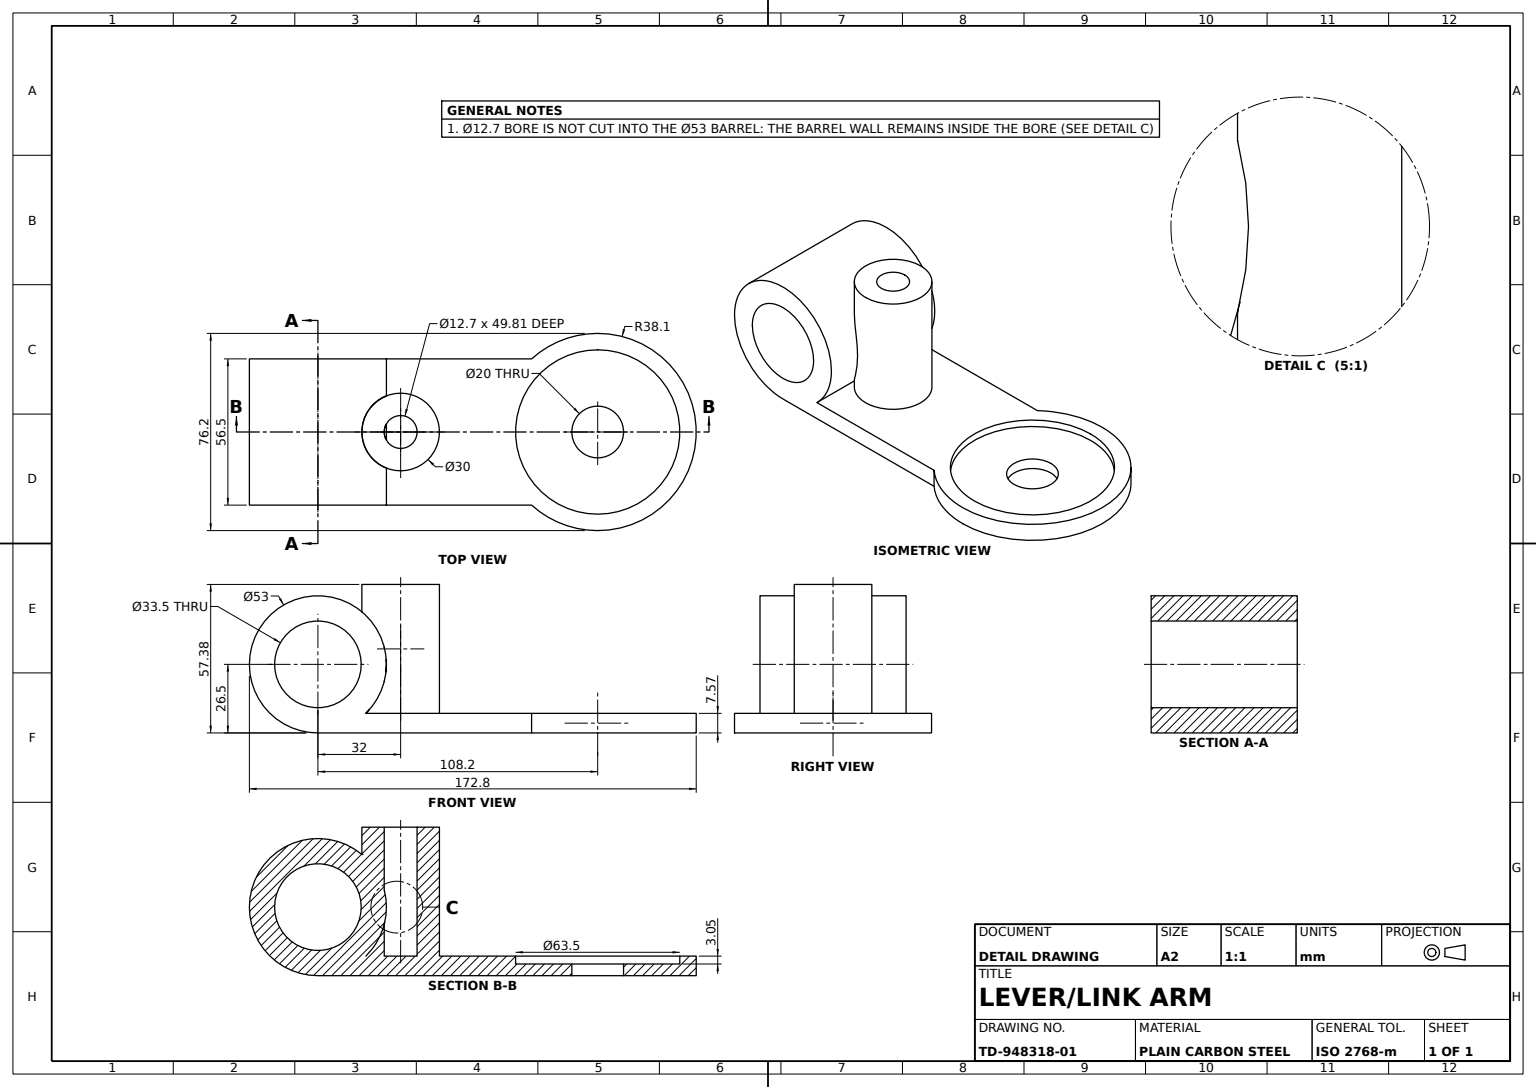
from build123d import *

# Parameters (mm, degrees)
PIVOT_TUBE_SKETCH_R       = 26.5
PIVOT_TUBE_SKETCH_R_2     = 16.75
PIVOT_TUBE_53X_33_5_DEPTH = 28.25
ARM_PLATE_DEPTH           = 28.25
POST_SKETCH_R             = 38.1
POST_SKETCH_R_2           = 31.75
POST_BOSS_DEPTH           = 26.5
POST_TRIM_SKETCH_W        = 76.2
POST_TRIM_SKETCH_H        = 18.935
POST_TRIM_CUT_DEPTH       = 50
MOUNTING_PAD_SKETCH_R     = 31.75
MOUNTING_PAD_DEPTH        = 7.565
PAD_RECESS_SKETCH_R       = 31.75
PAD_RECESS_DEPTH          = 3.05
PAD_HOLE_SKETCH_R         = 10
PAD_HOLE_20_DEPTH         = 159.764275657
ARM_LINK_SKETCH_R         = 15
ARM_LINK_SKETCH_R_2       = 6.35
ARM_LINK_BOSS_DEPTH       = 49.815


with BuildPart() as part:
    # Pivot Tube Sketch → Pivot Tube Ø53xØ33.5 (new, symmetric)
    with BuildSketch(Plane.XY):
        Circle(PIVOT_TUBE_SKETCH_R)
        Circle(PIVOT_TUBE_SKETCH_R_2, mode=Mode.SUBTRACT)
    extrude(amount=PIVOT_TUBE_53X_33_5_DEPTH, both=True)

    # Arm Profile Sketch → Arm Plate (add, symmetric)
    with BuildSketch(Plane.XY):
        with BuildLine():
            Line((0, -26.5), (108.2, -26.5))
            Line((108.2, -26.5), (108.2, -18.935))
            Line((108.2, -18.935), (18.539573215, -18.935))
            ThreePointArc((18.539573215, -18.935), (10.011805531, -24.535968495), (0, -26.5))
        make_face()
    extrude(amount=ARM_PLATE_DEPTH, both=True)

    # Post Sketch → Post Boss (add)
    with BuildSketch(Plane(origin=(0, 0, 0), x_dir=(1, 0, 0), z_dir=(0, 1, 0))):
        with Locations(Location((108.2, 0, 0), (0, 0, 270))):
            Circle(POST_SKETCH_R)
        with Locations(Location((108.2, 0, 0), (0, 0, 270))):
            Circle(POST_SKETCH_R_2, mode=Mode.SUBTRACT)
    extrude(amount=-POST_BOSS_DEPTH)

    # Post Trim Sketch → Post Trim Cut (cut, symmetric)
    with BuildSketch(Plane.XY):
        with Locations((108.2, -9.4675)):
            Rectangle(POST_TRIM_SKETCH_W, POST_TRIM_SKETCH_H)
    extrude(amount=POST_TRIM_CUT_DEPTH, both=True, mode=Mode.SUBTRACT)

    # Mounting Pad Sketch → Mounting Pad (add)
    with BuildSketch(Plane(origin=(0, -18.935, 0), x_dir=(1, 0, 0), z_dir=(0, 1, 0))):
        with Locations((108.2, 0)):
            Circle(MOUNTING_PAD_SKETCH_R)
    extrude(amount=-MOUNTING_PAD_DEPTH)

    # Pad Recess Sketch → Pad Recess (cut)
    with BuildSketch(Plane(origin=(0, -18.935, 0), x_dir=(1, 0, 0), z_dir=(0, 1, 0))):
        with Locations(Location((108.2, 0, 0), (0, 0, 270))):
            Circle(PAD_RECESS_SKETCH_R)
    extrude(amount=-PAD_RECESS_DEPTH, mode=Mode.SUBTRACT)

    # Pad Hole Sketch → Pad Hole Ø20 (cut, through all)
    with BuildSketch(Plane(origin=(0, -21.985, 0), x_dir=(1, 0, 0), z_dir=(0, 1, 0))):
        with Locations(Location((108.2, 0, 0), (0, 0, 270))):
            Circle(PAD_HOLE_SKETCH_R)
    extrude(amount=-PAD_HOLE_20_DEPTH, mode=Mode.SUBTRACT)

    # Arm Link Sketch → Arm Link Boss (add)
    with BuildSketch(Plane(origin=(0, -18.935, 0), x_dir=(1, 0, 0), z_dir=(0, 1, 0))):
        with Locations(Location((32, 0, 0), (0, 0, 153.813423855))):
            Circle(ARM_LINK_SKETCH_R)
        with Locations(Location((32, 0, 0), (0, 0, 270))):
            Circle(ARM_LINK_SKETCH_R_2, mode=Mode.SUBTRACT)
    extrude(amount=ARM_LINK_BOSS_DEPTH)


solid = part.part
